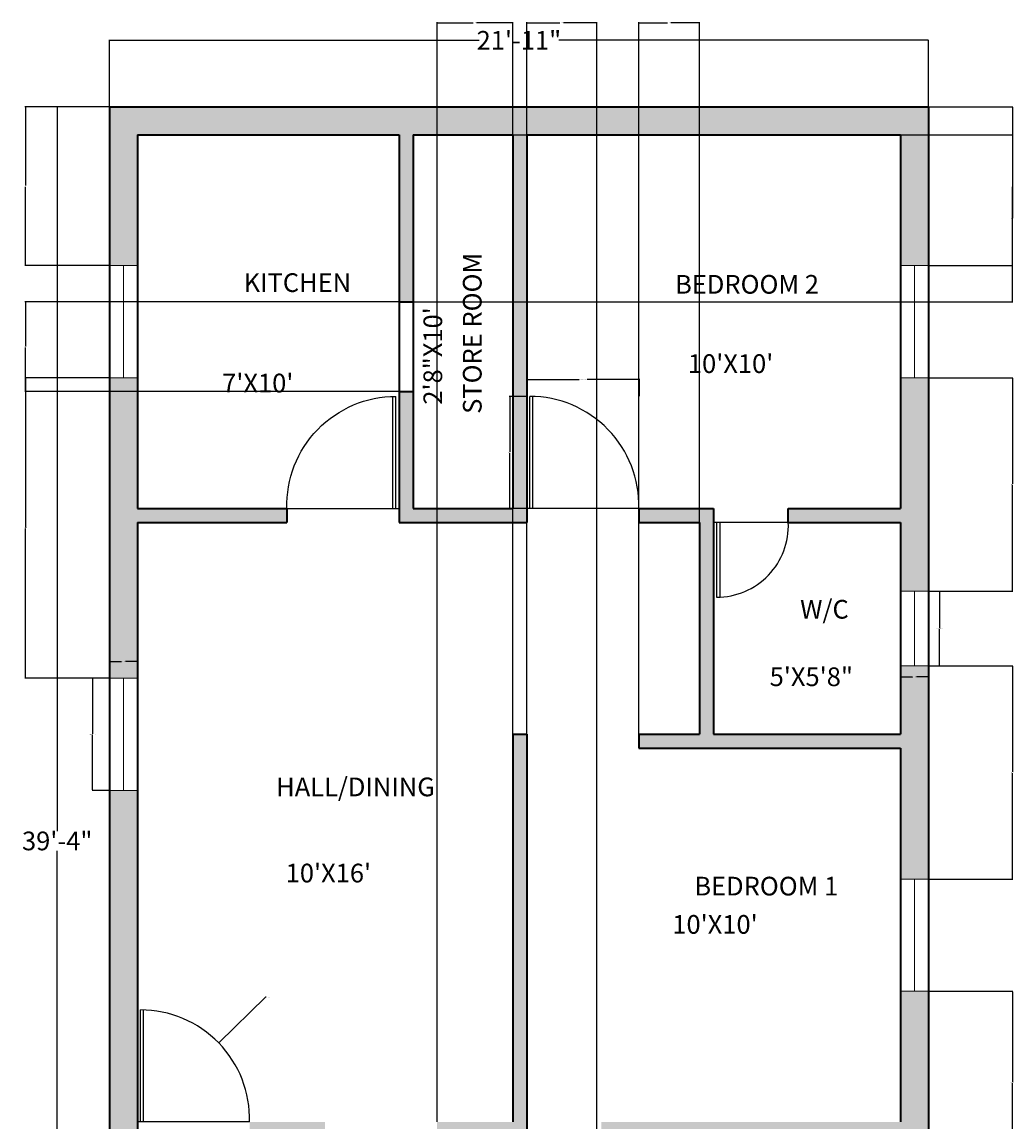
# Model space of a CAD drawing. Units: inches. Extents: x 2 to 321, y -521 to 41.
# Tile 2 of 2: x 2 to 321, y -312 to 41. Entities that reach past the tile are written whole.
import ezdxf

# ---------------------------------------------------------------- set-up
doc = ezdxf.new("R2010")
doc.units = ezdxf.units.IN
doc.header["$MEASUREMENT"] = 0
for name, color, linetype, lineweight in [('A-ANNO-DIMS', 2, 'Continuous', 18), ('A-ANNO-TEXT', 22, 'Continuous', 18), ('A-AREA-IDEN', 102, 'Continuous', 25), ('A-DOOR', 3, 'Continuous', 25), ('A-GLAZ', 4, 'Continuous', 18), ('A-WALL', 7, 'Continuous', 35), ('A-WALL-PATT', 5, 'Continuous', 13)]:
    doc.layers.add(name, color=color, linetype=linetype, lineweight=lineweight)
doc.styles.get("Standard").update_dxf_attribs({"font": 'arial.ttf'})
doc.dimstyles.get("Standard").update_dxf_attribs({"dimtxt": 0.18, "dimasz": 0.18, "dimexe": 0.18, "dimexo": 0.0625, "dimgap": 0.09, "dimtad": 0, "dimtih": 1, "dimtoh": 1, "dimdec": 0, "dimzin": 0, "dimdsep": 46, "dimlunit": 3, "dimtxsty": 'Standard', "dimcen": 0.09, "dimadec": 0, "dimazin": 0, "dimtfac": 1, "dimtdec": 0, "dimtofl": 0, "dimtmove": 0, "dimatfit": 3, "dimfxl": 1, "dimtolj": 1, "dimtzin": 0, "dimarcsym": 0})

# ---------------------------------------------------------------- blocks, each defined once
blk = doc.blocks.new('*D1')
at = {"layer": 'A-ANNO-DIMS', "color": 0, "lineweight": -2, "transparency": 16777216}
for p, q in [((30.16, 14.1), (30.16, 35.55)), ((30.34, 35.37), (148.88, 35.37)), ((292.98, 35.37), (174.44, 35.37)), ((293.16, 14.1), (293.16, 35.55))]:
    blk.add_line(p, q, dxfattribs=at)
at = {"layer": 'A-ANNO-DIMS', "color": 0, "transparency": 16777216}
for points in [[(30.34, 35.4), (30.34, 35.34), (30.16, 35.37)], [(292.98, 35.4), (292.98, 35.34), (293.16, 35.37)]]:
    blk.add_solid(points, dxfattribs=at)
at = {"layer": 'Defpoints', "color": 0, "transparency": 16777216}
for p in [(293.16, 35.37), (30.16, 14.04), (293.16, 14.04)]:
    blk.add_point(p, dxfattribs=at)
at = {"layer": 'A-ANNO-DIMS', "color": 0, "transparency": 16777216, "insert": (161.66, 35.37), "char_height": 6, "attachment_point": 5}
blk.add_mtext('\\A1;21\'-11"', dxfattribs=at)
blk = doc.blocks.new('*D2')
at = {"layer": 'A-ANNO-DIMS', "color": 0, "lineweight": -2, "transparency": 16777216}
for p, q in [((30.1, 14.04), (13.23, 14.04)), ((13.41, 13.86), (13.41, -218.56)), ((13.41, -457.28), (13.41, -224.87)), ((30.1, -457.46), (13.23, -457.46))]:
    blk.add_line(p, q, dxfattribs=at)
at = {"layer": 'A-ANNO-DIMS', "color": 0, "transparency": 16777216}
for points in [[(13.38, 13.86), (13.44, 13.86), (13.41, 14.04)], [(13.38, -457.28), (13.44, -457.28), (13.41, -457.46)]]:
    blk.add_solid(points, dxfattribs=at)
at = {"layer": 'Defpoints', "color": 0, "transparency": 16777216}
for p in [(30.16, 14.04), (13.41, -457.46), (30.16, -457.46)]:
    blk.add_point(p, dxfattribs=at)
at = {"layer": 'A-ANNO-DIMS', "color": 0, "transparency": 16777216, "insert": (13.41, -221.71), "char_height": 6, "attachment_point": 5}
blk.add_mtext('\\A1;39\'-4"', dxfattribs=at)
blk = doc.blocks.new('WIN-36IN-9IN-WALL')
for p, q in [((0, 36), (0, 0)), ((9, 36), (0, 36)), ((4.5, 36), (4.5, 0)), ((9, 0), (9, 36)), ((0, 0), (9, 0))]:
    blk.add_line(p, q)
blk = doc.blocks.new('WIN-24IN-9IN-WALL')
for p, q in [((0, 24), (0, 0)), ((9, 24), (0, 24)), ((4.5, 24), (4.5, 0)), ((9, 0), (9, 24)), ((0, 0), (9, 0))]:
    blk.add_line(p, q)
blk = doc.blocks.new('DOOR-SINGLE-36IN')
for p, q in [((1, 0), (1, 36)), ((2, 0), (2, 36)), ((36, 0), (0, 0))]:
    blk.add_line(p, q)
blk.add_arc((1, 0.99), 35.01, 358.3861, 90)
blk = doc.blocks.new('DOOR-SINGLE-24IN')
for p, q in [((24, 24), (0, 24)), ((1, 24), (1, 0)), ((2, 24), (2, 0))]:
    blk.add_line(p, q)
blk.add_arc((1, 23.02), 23.02, 270, 2.4378)
blk = doc.blocks.new('*D8')
at = {"layer": 'A-ANNO-DIMS', "color": 0, "lineweight": -2, "transparency": 16777216}
for p, q in [((30.1, -169.49), (24.58, -169.49)), ((24.76, -169.67), (24.76, -187.31)), ((24.76, -205.31), (24.76, -187.67)), ((30.1, -205.49), (24.58, -205.49))]:
    blk.add_line(p, q, dxfattribs=at)
at = {"layer": 'A-ANNO-DIMS', "color": 0, "transparency": 16777216}
for points in [[(24.73, -169.67), (24.79, -169.67), (24.76, -169.49)], [(24.73, -205.31), (24.79, -205.31), (24.76, -205.49)]]:
    blk.add_solid(points, dxfattribs=at)
at = {"layer": 'Defpoints', "color": 0, "transparency": 16777216}
for p in [(30.16, -169.49), (24.76, -205.49), (30.16, -205.49)]:
    blk.add_point(p, dxfattribs=at)
at = {"layer": 'A-ANNO-DIMS', "color": 0, "transparency": 16777216, "insert": (24.76, -187.49), "char_height": 0.18, "attachment_point": 5}
blk.add_mtext('\\A1;WINDOW 3\'-0" TYP.', dxfattribs=at)
blk = doc.blocks.new('*D9')
at = {"layer": 'A-ANNO-DIMS', "color": 0, "lineweight": -2, "transparency": 16777216}
for p, q in [((30.16, -169.43), (30.16, -163.91)), ((30.34, -164.09), (34.02, -164.09)), ((38.98, -164.09), (35.3, -164.09)), ((39.16, -169.43), (39.16, -163.91))]:
    blk.add_line(p, q, dxfattribs=at)
at = {"layer": 'A-ANNO-DIMS', "color": 0, "transparency": 16777216}
for points in [[(30.34, -164.06), (30.34, -164.12), (30.16, -164.09)], [(38.98, -164.06), (38.98, -164.12), (39.16, -164.09)]]:
    blk.add_solid(points, dxfattribs=at)
at = {"layer": 'Defpoints', "color": 0, "transparency": 16777216}
for p in [(30.16, -164.09), (30.16, -169.49), (39.16, -169.49)]:
    blk.add_point(p, dxfattribs=at)
at = {"layer": 'A-ANNO-DIMS', "color": 0, "transparency": 16777216, "insert": (34.66, -164.09), "char_height": 0.18, "attachment_point": 5}
blk.add_mtext('\\A1;0\'-9" TYP.', dxfattribs=at)
blk = doc.blocks.new('*D10')
at = {"layer": 'A-ANNO-DIMS', "color": 0, "lineweight": -2, "transparency": 16777216}
for p, q in [((293.22, -141.46), (296.94, -141.46)), ((296.76, -141.64), (296.76, -153.28)), ((296.76, -165.28), (296.76, -153.65)), ((293.22, -165.46), (296.94, -165.46))]:
    blk.add_line(p, q, dxfattribs=at)
at = {"layer": 'A-ANNO-DIMS', "color": 0, "transparency": 16777216}
for points in [[(296.73, -141.64), (296.79, -141.64), (296.76, -141.46)], [(296.73, -165.28), (296.79, -165.28), (296.76, -165.46)]]:
    blk.add_solid(points, dxfattribs=at)
at = {"layer": 'Defpoints', "color": 0, "transparency": 16777216}
for p in [(293.16, -141.46), (296.76, -141.46), (293.16, -165.46)]:
    blk.add_point(p, dxfattribs=at)
at = {"layer": 'A-ANNO-DIMS', "color": 0, "transparency": 16777216, "insert": (296.76, -153.46), "char_height": 0.18, "attachment_point": 5}
blk.add_mtext('\\A1;WINDOW 2\'-0" TYP.', dxfattribs=at)
blk = doc.blocks.new('*D11')
at = {"layer": 'A-ANNO-DIMS', "color": 0, "lineweight": -2, "transparency": 16777216}
for p, q in [((284.16, -165.53), (284.16, -169.24)), ((293.16, -165.53), (293.16, -169.24)), ((284.34, -169.06), (288.02, -169.06)), ((292.98, -169.06), (289.3, -169.06))]:
    blk.add_line(p, q, dxfattribs=at)
at = {"layer": 'A-ANNO-DIMS', "color": 0, "transparency": 16777216}
for points in [[(284.34, -169.03), (284.34, -169.09), (284.16, -169.06)], [(292.98, -169.03), (292.98, -169.09), (293.16, -169.06)]]:
    blk.add_solid(points, dxfattribs=at)
at = {"layer": 'Defpoints', "color": 0, "transparency": 16777216}
for p in [(284.16, -165.46), (293.16, -165.46), (293.16, -169.06)]:
    blk.add_point(p, dxfattribs=at)
at = {"layer": 'A-ANNO-DIMS', "color": 0, "transparency": 16777216, "insert": (288.66, -169.06), "char_height": 0.18, "attachment_point": 5}
blk.add_mtext('\\A1;0\'-9" TYP.', dxfattribs=at)
blk = doc.blocks.new('*D14')
at = {"layer": 'A-ANNO-DIMS', "color": 0, "lineweight": -2, "transparency": 16777216}
for p, q in [((164.16, -78.9), (164.16, -73.34)), ((164.34, -73.52), (181.04, -73.52)), ((200.25, -73.52), (183.55, -73.52)), ((200.43, -78.9), (200.43, -73.34))]:
    blk.add_line(p, q, dxfattribs=at)
at = {"layer": 'A-ANNO-DIMS', "color": 0, "transparency": 16777216}
for points in [[(164.34, -73.49), (164.34, -73.55), (164.16, -73.52)], [(200.25, -73.49), (200.25, -73.55), (200.43, -73.52)]]:
    blk.add_solid(points, dxfattribs=at)
at = {"layer": 'Defpoints', "color": 0, "transparency": 16777216}
for p in [(200.43, -73.52), (164.16, -78.96), (200.43, -78.96)]:
    blk.add_point(p, dxfattribs=at)
at = {"layer": 'A-ANNO-DIMS', "color": 0, "transparency": 16777216, "insert": (182.29, -73.52), "char_height": 0.18, "attachment_point": 5}
blk.add_mtext('\\A1;DOOR 3\'-0 1/2" TYP.', dxfattribs=at)
blk = doc.blocks.new('*D15')
at = {"layer": 'A-ANNO-DIMS', "color": 0, "lineweight": -2, "transparency": 16777216}
for p, q in [((164.1, -78.96), (158.54, -78.96)), ((158.72, -79.14), (158.72, -96.78)), ((158.72, -114.78), (158.72, -97.15)), ((164.1, -114.96), (158.54, -114.96))]:
    blk.add_line(p, q, dxfattribs=at)
at = {"layer": 'A-ANNO-DIMS', "color": 0, "transparency": 16777216}
for points in [[(158.69, -79.14), (158.75, -79.14), (158.72, -78.96)], [(158.69, -114.78), (158.75, -114.78), (158.72, -114.96)]]:
    blk.add_solid(points, dxfattribs=at)
at = {"layer": 'Defpoints', "color": 0, "transparency": 16777216}
for p in [(158.72, -78.96), (164.16, -78.96), (164.16, -114.96)]:
    blk.add_point(p, dxfattribs=at)
at = {"layer": 'A-ANNO-DIMS', "color": 0, "transparency": 16777216, "insert": (158.72, -96.96), "char_height": 0.18, "attachment_point": 5}
blk.add_mtext('\\A1;3\'-0" TYP.', dxfattribs=at)
blk = doc.blocks.new('*D21')
at = {"layer": 'A-ANNO-DIMS', "color": 0, "lineweight": -2, "transparency": 16777216}
for p, q in [((30.1, 14.04), (3.03, 14.04)), ((3.21, 13.86), (3.21, -11.28)), ((3.21, -36.78), (3.21, -11.65)), ((30.1, -36.96), (3.03, -36.96))]:
    blk.add_line(p, q, dxfattribs=at)
at = {"layer": 'A-ANNO-DIMS', "color": 0, "transparency": 16777216}
for points in [[(3.18, 13.86), (3.24, 13.86), (3.21, 14.04)], [(3.18, -36.78), (3.24, -36.78), (3.21, -36.96)]]:
    blk.add_solid(points, dxfattribs=at)
at = {"layer": 'Defpoints', "color": 0, "transparency": 16777216}
for p in [(30.16, 14.04), (3.21, -36.96), (30.16, -36.96)]:
    blk.add_point(p, dxfattribs=at)
at = {"layer": 'A-ANNO-DIMS', "color": 0, "transparency": 16777216, "insert": (3.21, -11.46), "char_height": 0.18, "attachment_point": 5}
blk.add_mtext('\\A1;4\'-3"', dxfattribs=at)
blk = doc.blocks.new('*D22')
at = {"layer": 'A-ANNO-DIMS', "color": 0, "lineweight": -2, "transparency": 16777216}
for p, q in [((30.1, -72.96), (3.03, -72.96)), ((3.21, -73.14), (3.21, -121.04)), ((3.21, -169.31), (3.21, -121.41)), ((30.1, -169.49), (3.03, -169.49))]:
    blk.add_line(p, q, dxfattribs=at)
at = {"layer": 'A-ANNO-DIMS', "color": 0, "transparency": 16777216}
for points in [[(3.18, -73.14), (3.24, -73.14), (3.21, -72.96)], [(3.18, -169.31), (3.24, -169.31), (3.21, -169.49)]]:
    blk.add_solid(points, dxfattribs=at)
at = {"layer": 'Defpoints', "color": 0, "transparency": 16777216}
for p in [(30.16, -72.96), (3.21, -169.49), (30.16, -169.49)]:
    blk.add_point(p, dxfattribs=at)
at = {"layer": 'A-ANNO-DIMS', "color": 0, "transparency": 16777216, "insert": (3.21, -121.23), "char_height": 0.18, "attachment_point": 5}
blk.add_mtext('\\A1;8\'-0 1/2"', dxfattribs=at)
blk = doc.blocks.new('*D23')
at = {"layer": 'A-ANNO-DIMS', "color": 0, "lineweight": -2, "transparency": 16777216}
for p, q in [((293.22, 14.04), (320.29, 14.04)), ((320.11, 13.86), (320.11, -11.28)), ((320.11, -36.78), (320.11, -11.65)), ((293.22, -36.96), (320.29, -36.96))]:
    blk.add_line(p, q, dxfattribs=at)
at = {"layer": 'A-ANNO-DIMS', "color": 0, "transparency": 16777216}
for points in [[(320.08, 13.86), (320.14, 13.86), (320.11, 14.04)], [(320.08, -36.78), (320.14, -36.78), (320.11, -36.96)]]:
    blk.add_solid(points, dxfattribs=at)
at = {"layer": 'Defpoints', "color": 0, "transparency": 16777216}
for p in [(293.16, 14.04), (293.16, -36.96), (320.11, -36.96)]:
    blk.add_point(p, dxfattribs=at)
at = {"layer": 'A-ANNO-DIMS', "color": 0, "transparency": 16777216, "insert": (320.11, -11.46), "char_height": 0.18, "attachment_point": 5}
blk.add_mtext('\\A1;4\'-3"', dxfattribs=at)
blk = doc.blocks.new('*D24')
at = {"layer": 'A-ANNO-DIMS', "color": 0, "lineweight": -2, "transparency": 16777216}
for p, q in [((293.22, -72.96), (320.29, -72.96)), ((320.11, -73.14), (320.11, -107.03)), ((320.11, -141.28), (320.11, -107.4)), ((293.22, -141.46), (320.29, -141.46))]:
    blk.add_line(p, q, dxfattribs=at)
at = {"layer": 'A-ANNO-DIMS', "color": 0, "transparency": 16777216}
for points in [[(320.08, -73.14), (320.14, -73.14), (320.11, -72.96)], [(320.08, -141.28), (320.14, -141.28), (320.11, -141.46)]]:
    blk.add_solid(points, dxfattribs=at)
at = {"layer": 'Defpoints', "color": 0, "transparency": 16777216}
for p in [(293.16, -72.96), (293.16, -141.46), (320.11, -141.46)]:
    blk.add_point(p, dxfattribs=at)
at = {"layer": 'A-ANNO-DIMS', "color": 0, "transparency": 16777216, "insert": (320.11, -107.21), "char_height": 0.18, "attachment_point": 5}
blk.add_mtext('\\A1;5\'-8 1/2"', dxfattribs=at)
blk = doc.blocks.new('*D25')
at = {"layer": 'A-ANNO-DIMS', "color": 0, "lineweight": -2, "transparency": 16777216}
for p, q in [((293.22, -165.46), (320.29, -165.46)), ((320.11, -165.64), (320.11, -199.53)), ((320.11, -233.78), (320.11, -199.9)), ((293.22, -233.96), (320.29, -233.96))]:
    blk.add_line(p, q, dxfattribs=at)
at = {"layer": 'A-ANNO-DIMS', "color": 0, "transparency": 16777216}
for points in [[(320.08, -165.64), (320.14, -165.64), (320.11, -165.46)], [(320.08, -233.78), (320.14, -233.78), (320.11, -233.96)]]:
    blk.add_solid(points, dxfattribs=at)
at = {"layer": 'Defpoints', "color": 0, "transparency": 16777216}
for p in [(293.16, -165.46), (293.16, -233.96), (320.11, -233.96)]:
    blk.add_point(p, dxfattribs=at)
at = {"layer": 'A-ANNO-DIMS', "color": 0, "transparency": 16777216, "insert": (320.11, -199.71), "char_height": 0.18, "attachment_point": 5}
blk.add_mtext('\\A1;5\'-8 1/2"', dxfattribs=at)
blk = doc.blocks.new('*D26')
at = {"layer": 'A-ANNO-DIMS', "color": 0, "lineweight": -2, "transparency": 16777216}
for p, q in [((293.22, -269.96), (320.29, -269.96)), ((320.11, -270.14), (320.11, -299.03)), ((320.11, -328.28), (320.11, -299.4)), ((293.22, -328.46), (320.29, -328.46))]:
    blk.add_line(p, q, dxfattribs=at)
at = {"layer": 'A-ANNO-DIMS', "color": 0, "transparency": 16777216}
for points in [[(320.08, -270.14), (320.14, -270.14), (320.11, -269.96)], [(320.08, -328.28), (320.14, -328.28), (320.11, -328.46)]]:
    blk.add_solid(points, dxfattribs=at)
at = {"layer": 'Defpoints', "color": 0, "transparency": 16777216}
for p in [(293.16, -269.96), (293.16, -328.46), (320.11, -328.46)]:
    blk.add_point(p, dxfattribs=at)
at = {"layer": 'A-ANNO-DIMS', "color": 0, "transparency": 16777216, "insert": (320.11, -299.21), "char_height": 0.18, "attachment_point": 5}
blk.add_mtext('\\A1;4\'-10 1/2"', dxfattribs=at)
blk = doc.blocks.new('*D29')
at = {"layer": 'A-ANNO-DIMS', "color": 0, "lineweight": -2, "transparency": 16777216}
for p, q in [((135.41, -311.9), (135.41, 41.17)), ((135.59, 40.99), (147, 40.99)), ((159.48, 40.99), (148.08, 40.99)), ((159.66, -311.9), (159.66, 41.17))]:
    blk.add_line(p, q, dxfattribs=at)
at = {"layer": 'A-ANNO-DIMS', "color": 0, "transparency": 16777216}
for points in [[(135.59, 41.02), (135.59, 40.96), (135.41, 40.99)], [(159.48, 41.02), (159.48, 40.96), (159.66, 40.99)]]:
    blk.add_solid(points, dxfattribs=at)
at = {"layer": 'Defpoints', "color": 0, "transparency": 16777216}
for p in [(159.66, 40.99), (135.41, -311.96), (159.66, -311.96)]:
    blk.add_point(p, dxfattribs=at)
at = {"layer": 'A-ANNO-DIMS', "color": 0, "transparency": 16777216, "insert": (147.54, 40.99), "char_height": 0.18, "attachment_point": 5}
blk.add_mtext('\\A1;2\'-0 1/2"', dxfattribs=at)
blk = doc.blocks.new('*D30')
at = {"layer": 'A-ANNO-DIMS', "color": 0, "lineweight": -2, "transparency": 16777216}
for p, q in [((164.16, -364.4), (164.16, 41.17)), ((164.34, 40.99), (174.81, 40.99)), ((186.48, 40.99), (176.01, 40.99)), ((186.66, -364.4), (186.66, 41.17))]:
    blk.add_line(p, q, dxfattribs=at)
at = {"layer": 'A-ANNO-DIMS', "color": 0, "transparency": 16777216}
for points in [[(164.34, 41.02), (164.34, 40.96), (164.16, 40.99)], [(186.48, 41.02), (186.48, 40.96), (186.66, 40.99)]]:
    blk.add_solid(points, dxfattribs=at)
at = {"layer": 'Defpoints', "color": 0, "transparency": 16777216}
for p in [(186.66, 40.99), (164.16, -364.46), (186.66, -364.46)]:
    blk.add_point(p, dxfattribs=at)
at = {"layer": 'A-ANNO-DIMS', "color": 0, "transparency": 16777216, "insert": (175.41, 40.99), "char_height": 0.18, "attachment_point": 5}
blk.add_mtext('\\A1;1\'-10 1/2"', dxfattribs=at)
blk = doc.blocks.new('*D34')
at = {"layer": 'A-ANNO-DIMS', "color": 0, "lineweight": -2, "transparency": 16777216}
for p, q in [((200.16, -187.4), (200.16, 41.17)), ((200.34, 40.99), (209.38, 40.99)), ((219.48, 40.99), (210.44, 40.99)), ((219.66, -187.4), (219.66, 41.17))]:
    blk.add_line(p, q, dxfattribs=at)
at = {"layer": 'A-ANNO-DIMS', "color": 0, "transparency": 16777216}
for points in [[(200.34, 41.02), (200.34, 40.96), (200.16, 40.99)], [(219.48, 41.02), (219.48, 40.96), (219.66, 40.99)]]:
    blk.add_solid(points, dxfattribs=at)
at = {"layer": 'Defpoints', "color": 0, "transparency": 16777216}
for p in [(219.66, 40.99), (200.16, -187.46), (219.66, -187.46)]:
    blk.add_point(p, dxfattribs=at)
at = {"layer": 'A-ANNO-DIMS', "color": 0, "transparency": 16777216, "insert": (209.91, 40.99), "char_height": 0.18, "attachment_point": 5}
blk.add_mtext('\\A1;1\'-7 1/2"', dxfattribs=at)
blk = doc.blocks.new('*D35')
at = {"layer": 'A-ANNO-DIMS', "color": 0, "lineweight": -2, "transparency": 16777216}
for p, q in [((123.1, -48.65), (3.03, -48.65)), ((3.21, -48.83), (3.21, -62.86)), ((3.21, -77.26), (3.21, -63.22)), ((123.1, -77.44), (3.03, -77.44))]:
    blk.add_line(p, q, dxfattribs=at)
at = {"layer": 'A-ANNO-DIMS', "color": 0, "transparency": 16777216}
for points in [[(3.18, -48.83), (3.24, -48.83), (3.21, -48.65)], [(3.18, -77.26), (3.24, -77.26), (3.21, -77.44)]]:
    blk.add_solid(points, dxfattribs=at)
at = {"layer": 'Defpoints', "color": 0, "transparency": 16777216}
for p in [(123.16, -48.65), (3.21, -77.44), (123.16, -77.44)]:
    blk.add_point(p, dxfattribs=at)
at = {"layer": 'A-ANNO-DIMS', "color": 0, "transparency": 16777216, "insert": (3.21, -63.04), "char_height": 0.18, "attachment_point": 5}
blk.add_mtext('\\A1;2\'-5"', dxfattribs=at)
blk = doc.blocks.new('*D36')
at = {"layer": 'A-ANNO-DIMS', "color": 0, "lineweight": -2, "transparency": 16777216}
for p, q in [((127.72, 5.04), (320.29, 5.04)), ((320.11, 4.86), (320.11, -21.62)), ((320.11, -48.47), (320.11, -21.99)), ((127.72, -48.65), (320.29, -48.65))]:
    blk.add_line(p, q, dxfattribs=at)
at = {"layer": 'A-ANNO-DIMS', "color": 0, "transparency": 16777216}
for points in [[(320.08, 4.86), (320.14, 4.86), (320.11, 5.04)], [(320.08, -48.47), (320.14, -48.47), (320.11, -48.65)]]:
    blk.add_solid(points, dxfattribs=at)
at = {"layer": 'Defpoints', "color": 0, "transparency": 16777216}
for p in [(127.66, 5.04), (127.66, -48.65), (320.11, -48.65)]:
    blk.add_point(p, dxfattribs=at)
at = {"layer": 'A-ANNO-DIMS', "color": 0, "transparency": 16777216, "insert": (320.11, -21.81), "char_height": 0.18, "attachment_point": 5}
blk.add_mtext('\\A1;4\'-5 1/2"', dxfattribs=at)
blk = doc.blocks.new('*D38')
at = {"layer": 'A-ANNO-DIMS', "color": 0, "lineweight": -2, "transparency": 16777216}
for p, q in [((80.33, -271.93), (65.39, -286.44)), ((80.51, -271.93), (80.33, -271.93)), ((40.07, -310.98), (40.25, -310.98)), ((40.16, -311.07), (40.16, -310.89))]:
    blk.add_line(p, q, dxfattribs=at)
at = {"layer": 'A-ANNO-DIMS', "color": 0, "transparency": 16777216}
blk.add_solid([(65.37, -286.42), (65.41, -286.47), (65.27, -286.57)], dxfattribs=at)
at = {"layer": 'Defpoints', "color": 0, "transparency": 16777216}
for p in [(65.27, -286.57), (40.16, -310.98)]:
    blk.add_point(p, dxfattribs=at)
at = {"layer": 'A-ANNO-DIMS', "color": 0, "transparency": 16777216, "insert": (81.19, -271.93), "char_height": 0.18, "attachment_point": 5}
blk.add_mtext('\\A1;2X R2\'-11"', dxfattribs=at)

msp = doc.modelspace()

# ---------------------------------------------------------------- hatches: boundary and pattern name
at = {"layer": 'A-WALL-PATT'}
h = msp.add_hatch(color=256, dxfattribs=at)
h.dxf.hatch_style = 1
h.paths.add_polyline_path([(39.16, 5.04), (123.16, 5.04), (123.16, -48.65), (127.66, -48.65), (127.66, 5.04), (159.66, 5.04), (159.66, -114.96), (127.66, -114.96), (127.66, -77.44), (123.16, -77.44), (123.16, -119.46), (164.16, -119.46), (164.16, 5.04), (284.16, 5.04), (284.16, -36.96), (293.16, -36.96), (293.16, 14.04), (30.16, 14.04), (30.16, -36.96), (39.16, -36.96)])
h.paths.add_polyline_path([(39.16, -205.49), (30.16, -205.49), (30.16, -457.46), (46.07, -457.46), (46.07, -448.46), (39.16, -448.46)])
h.paths.add_polyline_path([(39.16, -119.46), (87.16, -119.46), (87.16, -114.96), (39.16, -114.96), (39.16, -72.96), (30.16, -72.96), (30.16, -169.49), (39.16, -169.49)])
h.paths.add_polyline_path([(293.16, -165.46), (284.16, -165.46), (284.16, -187.46), (224.16, -187.46), (224.16, -114.96), (200.16, -114.96), (200.16, -119.46), (219.66, -119.46), (219.66, -187.46), (200.16, -187.46), (200.16, -191.96), (284.16, -191.96), (284.16, -233.96), (293.16, -233.96)])
h.paths.add_polyline_path([(293.16, -72.96), (284.16, -72.96), (284.16, -114.96), (248.16, -114.96), (248.16, -119.46), (284.16, -119.46), (284.16, -141.46), (293.16, -141.46)])
h.paths.add_polyline_path([(293.16, -269.96), (284.16, -269.96), (284.16, -311.96), (188.16, -311.96), (188.16, -316.46), (231.66, -316.46), (231.66, -364.46), (222.66, -364.46), (222.66, -368.96), (260.16, -368.96), (260.16, -364.46), (236.16, -364.46), (236.16, -316.46), (284.16, -316.46), (284.16, -328.46), (293.16, -328.46)])
h.paths.add_polyline_path([(186.66, -364.46), (164.16, -364.46), (164.16, -187.46), (159.66, -187.46), (159.66, -311.96), (135.41, -311.96), (135.41, -316.46), (159.66, -316.46), (159.66, -368.96), (186.66, -368.96)])
h.paths.add_polyline_path([(293.16, -426.71), (284.16, -426.71), (284.16, -448.46), (118.07, -448.46), (118.07, -457.46), (293.16, -457.46)])
h.paths.add_polyline_path([(99.41, -311.96), (75.16, -311.96), (75.16, -316.46), (99.41, -316.46)])
h.paths.add_polyline_path([(293.16, -352.46), (284.16, -352.46), (284.16, -364.46), (284.16, -368.96), (284.16, -390.71), (293.16, -390.71)])

# ---------------------------------------------------------------- linework, layer by layer
at = {"layer": 'A-WALL'}
for p, q in [((30.16, 14.04), (30.16, -457.46)), ((30.16, 14.04), (293.16, 14.04)), ((293.16, 14.04), (293.16, -457.46)), ((39.16, 5.04), (39.16, -114.96)), ((39.16, 5.04), (123.16, 5.04)), ((123.16, 5.04), (123.16, -119.46)), ((127.66, 5.04), (127.66, -114.96)), ((127.66, 5.04), (159.66, 5.04)), ((159.66, 5.04), (159.66, -114.96)), ((164.16, 5.04), (164.16, -119.46)), ((164.16, 5.04), (284.16, 5.04)), ((284.16, 5.04), (284.16, -114.96)), ((123.16, -48.65), (127.66, -48.65)), ((123.16, -77.44), (127.66, -77.44)), ((39.16, -114.96), (87.16, -114.96)), ((87.16, -114.96), (87.16, -119.46)), ((127.66, -114.96), (159.66, -114.96)), ((200.16, -114.96), (224.16, -114.96)), ((200.16, -114.96), (200.16, -119.46)), ((224.16, -114.96), (224.16, -187.46)), ((248.16, -119.46), (248.16, -114.96)), ((248.16, -114.96), (284.16, -114.96)), ((39.16, -119.46), (87.16, -119.46)), ((39.16, -119.46), (39.16, -448.46)), ((123.16, -119.46), (164.16, -119.46)), ((200.16, -119.46), (219.66, -119.46)), ((219.66, -119.46), (219.66, -187.46)), ((248.16, -119.46), (284.16, -119.46)), ((284.16, -119.46), (284.16, -187.46)), ((159.66, -187.46), (164.16, -187.46)), ((159.66, -187.46), (159.66, -311.96)), ((164.16, -187.46), (164.16, -364.46)), ((200.16, -187.46), (200.16, -191.96)), ((200.16, -187.46), (219.66, -187.46)), ((224.16, -187.46), (284.16, -187.46)), ((200.16, -191.96), (284.16, -191.96)), ((284.16, -191.96), (284.16, -311.96))]:
    msp.add_line(p, q, dxfattribs=at)

# ---------------------------------------------------------------- block references
at = {"layer": 'A-DOOR', "extrusion": (0, 0, -1), "zscale": -1}
msp.add_blockref('DOOR-SINGLE-36IN', (-123.16, -114.96), dxfattribs=at)
at = {"layer": 'A-DOOR'}
for name, p in [('DOOR-SINGLE-36IN', (164.16, -114.96)), ('DOOR-SINGLE-24IN', (224.16, -143.46)), ('DOOR-SINGLE-36IN', (39.16, -311.96))]:
    msp.add_blockref(name, p, dxfattribs=at)
at = {"layer": 'A-GLAZ'}
for name, p in [('WIN-36IN-9IN-WALL', (30.16, -72.96)), ('WIN-24IN-9IN-WALL', (284.16, -165.46))]:
    msp.add_blockref(name, p, dxfattribs=at)
at = {"layer": 'A-GLAZ', "rotation": 180}
for p in [(293.16, -36.96), (39.16, -169.49), (293.16, -233.96)]:
    msp.add_blockref('WIN-36IN-9IN-WALL', p, dxfattribs=at)

# ---------------------------------------------------------------- texts
at = {"layer": 'A-ANNO-TEXT', "insert": (131.02, -81.62), "char_height": 6, "attachment_point": 1, "rotation": 90}
msp.add_mtext('2\'8"X10\'', dxfattribs=at)
at = {"layer": 'A-ANNO-TEXT', "char_height": 6, "attachment_point": 1}
for s, insert in [("10'X10'", (215.93, -65.45)), ("7'X10'", (66.38, -71.68)), ('5\'X5\'8"', (242.18, -165.99)), ("10'X16'", (86.78, -229.03)), ("10'X10'", (210.93, -245.51))]:
    msp.add_mtext(s, dxfattribs=dict(at, insert=insert))
at = {"layer": 'A-AREA-IDEN', "insert": (143.69, -84.57), "char_height": 6, "attachment_point": 1, "rotation": 90}
msp.add_mtext_dynamic_manual_height_columns('STORE ROOM ', width=77.4807, gutter_width=1, heights=[9.94], dxfattribs=at)
at = {"layer": 'A-AREA-IDEN', "char_height": 6, "attachment_point": 1}
for s, insert in [('KITCHEN', (73.26, -39.44)), ('BEDROOM 2', (211.82, -39.98)), ('W/C', (251.96, -144.33)), ('HALL/DINING', (83.72, -201.37)), ('BEDROOM 1', (218, -233.22))]:
    msp.add_mtext(s, dxfattribs=dict(at, insert=insert))

# ---------------------------------------------------------------- dimensions: what is measured, and where the dimension line sits
at = {"layer": 'A-ANNO-DIMS'}
for base, p1, p2, override, picture, middle in [((293.16, 35.37), (30.16, 14.04), (293.16, 14.04), {"dimtxt": 6, "dimclrd": 0, "dimclre": 0, "dimclrt": 0}, '*D1', (161.66, 35.37)), ((159.660635, 40.986053), (135.410635, -311.963947), (159.660635, -311.963947), {"dimdec": 1, "dimlfac": 1, "dimrnd": 0, "dimzin": 1, "dimdsep": 46, "dimlunit": 4, "dimfrac": 2}, '*D29', (147.535635, 40.986053)), ((186.66, 40.99), (164.16, -364.46), (186.66, -364.46), {"dimdec": 1, "dimlfac": 1, "dimrnd": 0, "dimzin": 1, "dimdsep": 46, "dimlunit": 4, "dimfrac": 2}, '*D30', (175.41, 40.99)), ((219.66, 40.99), (200.16, -187.46), (219.66, -187.46), {"dimdec": 1, "dimlfac": 1, "dimrnd": 0, "dimzin": 1, "dimdsep": 46, "dimlunit": 4, "dimfrac": 2}, '*D34', (209.91, 40.99))]:
    dim = msp.add_linear_dim(base=base, p1=p1, p2=p2, dimstyle='Standard', override=override, dxfattribs=at)
    dim.commit()
    dim.dimension.update_dxf_attribs({"geometry": picture, "text_midpoint": middle})
for base, p1, p2, override, picture, middle in [((13.41474495, -457.46394712), (30.16063488, 14.03605288), (30.16063488, -457.46394712), {"dimtxt": 6, "dimclrd": 0, "dimclre": 0, "dimclrt": 0}, '*D2', (13.41474495, -221.71394712)), ((3.21, -36.96), (30.16, 14.04), (30.16, -36.96), {"dimdec": 1, "dimlfac": 1, "dimrnd": 0, "dimzin": 1, "dimdsep": 46, "dimlunit": 4, "dimfrac": 2}, '*D21', (3.21, -11.46)), ((320.11, -36.96), (293.16, 14.04), (293.16, -36.96), {"dimdec": 1, "dimlfac": 1, "dimrnd": 0, "dimzin": 1, "dimdsep": 46, "dimlunit": 4, "dimfrac": 2}, '*D23', (320.11, -11.46)), ((320.11, -48.65), (127.66, 5.04), (127.66, -48.65), {"dimdec": 1, "dimlfac": 1, "dimrnd": 0, "dimzin": 1, "dimdsep": 46, "dimlunit": 4, "dimfrac": 2}, '*D36', (320.11, -21.81)), ((3.21, -77.44), (123.16, -48.65), (123.16, -77.44), {"dimdec": 1, "dimlfac": 1, "dimrnd": 0, "dimzin": 1, "dimdsep": 46, "dimlunit": 4, "dimfrac": 2}, '*D35', (3.21, -63.04)), ((3.21, -169.49), (30.16, -72.96), (30.16, -169.49), {"dimdec": 1, "dimlfac": 1, "dimrnd": 0, "dimzin": 1, "dimdsep": 46, "dimlunit": 4, "dimfrac": 2}, '*D22', (3.21, -121.23)), ((320.11, -141.46), (293.16, -72.96), (293.16, -141.46), {"dimdec": 1, "dimlfac": 1, "dimrnd": 0, "dimzin": 1, "dimdsep": 46, "dimlunit": 4, "dimfrac": 2}, '*D24', (320.11, -107.21)), ((320.11, -233.96), (293.16, -165.46), (293.16, -233.96), {"dimdec": 1, "dimlfac": 1, "dimrnd": 0, "dimzin": 1, "dimdsep": 46, "dimlunit": 4, "dimfrac": 2}, '*D25', (320.11, -199.71)), ((320.11, -328.46), (293.16, -269.96), (293.16, -328.46), {"dimdec": 1, "dimlfac": 1, "dimrnd": 0, "dimzin": 1, "dimdsep": 46, "dimlunit": 4, "dimfrac": 2}, '*D26', (320.11, -299.21))]:
    dim = msp.add_linear_dim(base=base, p1=p1, p2=p2, angle=90, dimstyle='Standard', override=override, dxfattribs=at)
    dim.commit()
    dim.dimension.update_dxf_attribs({"geometry": picture, "text_midpoint": middle})
for base, p1, p2, text, picture, middle in [((200.43, -73.52), (164.16, -78.96), (200.43, -78.96), 'DOOR <> TYP.', '*D14', (182.29, -73.52)), ((293.16, -169.06), (284.16, -165.46), (293.16, -165.46), '<> TYP.', '*D11', (288.66, -169.06))]:
    dim = msp.add_linear_dim(base=base, p1=p1, p2=p2, text=text, dimstyle='Standard', override={"dimdec": 1, "dimlfac": 1, "dimrnd": 0, "dimzin": 1, "dimdsep": 46, "dimlunit": 4, "dimfrac": 2}, dxfattribs=at)
    dim.commit()
    dim.dimension.update_dxf_attribs({"geometry": picture, "text_midpoint": middle})
for base, p1, p2, angle, text, picture, middle in [((158.72, -78.96), (164.16, -114.96), (164.16, -78.96), 90, '<> TYP.', '*D15', (158.72, -96.96)), ((296.76, -141.46), (293.16, -165.46), (293.16, -141.46), 90, 'WINDOW <> TYP.', '*D10', (296.76, -153.46)), ((30.16, -164.09), (39.16, -169.49), (30.16, -169.49), 180, '<> TYP.', '*D9', (34.66, -164.09)), ((24.76, -205.49), (30.16, -169.49), (30.16, -205.49), 270, 'WINDOW <> TYP.', '*D8', (24.76, -187.49))]:
    dim = msp.add_linear_dim(base=base, p1=p1, p2=p2, angle=angle, text=text, dimstyle='Standard', override={"dimdec": 1, "dimlfac": 1, "dimrnd": 0, "dimzin": 1, "dimdsep": 46, "dimlunit": 4, "dimfrac": 2}, dxfattribs=at)
    dim.commit()
    dim.dimension.update_dxf_attribs({"geometry": picture, "text_midpoint": middle})
dim = msp.add_radius_dim(center=(40.16, -310.98), mpoint=(65.27, -286.57), text='2X <>', dimstyle='Standard', override={"dimdec": 1, "dimlfac": 1, "dimrnd": 0, "dimzin": 1, "dimdsep": 46, "dimlunit": 4, "dimfrac": 2}, dxfattribs=at)
dim.commit()
dim.dimension.update_dxf_attribs({"geometry": '*D38', "text_midpoint": (81.19, -271.93), "dimtype": 164})

doc.saveas('drawing.dxf')
